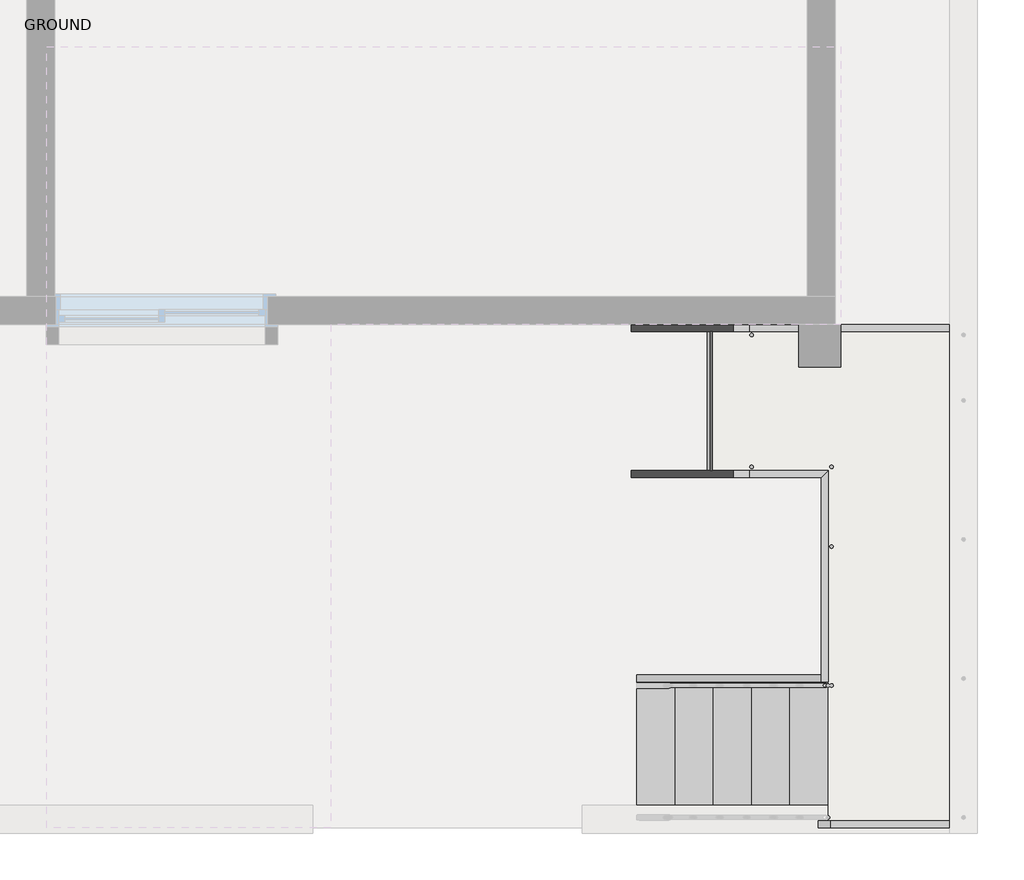
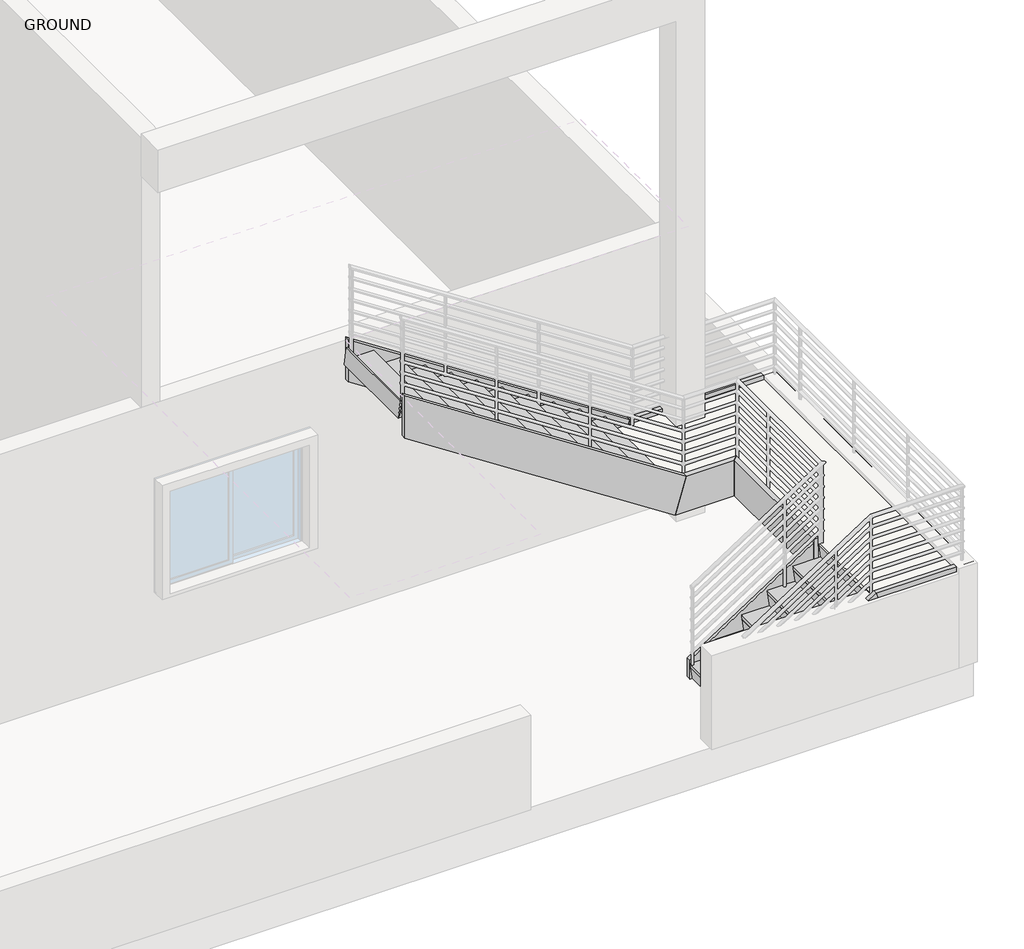
# One storey, part 4 of 4: 9 members, 2 stair flights, 1 slab.
"""IFC4 building model written with IfcOpenShell, lengths in millimetres."""

from ifc_helpers import new_model, si_unit, frame, origin, place, context, project, spatial, polyline, outline, extrude, faceted_brep, transform, mapped, element, save
from components import non_monolithic_landing_a96adf93, stair_flight_50mm_tread_25mm_nosing_13mm_riser_d89b79ae, stair_flight_50mm_tread_25mm_nosing_13mm_riser_9fd7d1ab

model = new_model("IFC4")

# Units and contexts
model_context = context("Model", 3, world=origin())
ifc_project = project(units=[si_unit("LENGTHUNIT", "METRE", prefix="MILLI")], contexts=[model_context])

# Site, building, storey
site = spatial("IfcSite", under=ifc_project)
building = spatial("IfcBuilding", under=site)
storey = spatial("IfcBuildingStorey", under=building, Name="GROUND", Elevation=0.0)

# Members
placement = place(None, origin())
element("IfcMember", 1, ObjectType="Stringer - 50mm Width", at=placement, inside=storey, context=model_context, shape_type="SweptSolid", body=[
    extrude(outline(polyline([(216.9803521, 11825.7864069), (0.0, 11825.7864069), (0.0, 12225.3790476), (603.3458035, 13150.7864069), (1080.8520099, 13150.7864069), (216.9803521, 11825.7864069)])), frame((0.0, -2533.727917, 0.0), z_axis=(0.0, 1.0, 0.0), x_axis=(0.0, 0.0, 1.0)), (0.0, 0.0, 1.0), 50.0),
])
element("IfcMember", 2, ObjectType="Stringer - 50mm Width", at=placement, inside=storey, context=model_context, shape_type="SweptSolid", body=[
    extrude(outline(polyline([(216.9803521, 11825.7864069), (0.0, 11825.7864069), (0.0, 12225.3790476), (723.1584328, 13334.5541373), (1123.1584328, 13215.6756875), (216.9803521, 11825.7864069)])), frame((0.0, -3583.7536983, 0.0), z_axis=(0.0, 1.0, 0.0), x_axis=(0.0, 0.0, 1.0)), (0.0, 0.0, 1.0), 50.0),
])
element("IfcMember", 3, ObjectType="Stringer - 50mm Width", at=placement, inside=storey, context=model_context, shape_type="SweptSolid", body=[
    extrude(outline(polyline([(723.1584328, 12517.0186765), (1123.1584328, 12635.8971263), (3085.6862345, 9625.7864069), (2608.1800281, 9625.7864069), (723.1584328, 12517.0186765)])), frame((0.0, -1061.9101069, 0.0), z_axis=(0.0, 1.0, 0.0), x_axis=(0.0, 0.0, 1.0)), (0.0, 0.0, 1.0), 50.0),
])
element("IfcMember", 4, ObjectType="Stringer - 50mm Width", at=placement, inside=storey, context=model_context, shape_type="SweptSolid", body=[
    extrude(outline(polyline([(723.1584328, 12517.0186765), (1123.1584328, 12635.8971263), (3085.6862345, 9625.7864069), (2608.1800281, 9625.7864069), (723.1584328, 12517.0186765)])), frame((0.0, -11.8843256, 0.0), z_axis=(0.0, 1.0, 0.0), x_axis=(0.0, 0.0, 1.0)), (0.0, 0.0, 1.0), 50.0),
])
element("IfcMember", 5, ObjectType="Stringer - 50mm Width", at=placement, inside=storey, context=model_context, shape_type="Brep", body=[
    faceted_brep([(12635.8971263, -1011.9101069, 1123.1584328), (12635.8971263, -1061.9101069, 1123.1584328), (13150.7864069, -1061.9101069, 1123.1584328), (13200.7864069, -1011.9101069, 1123.1584328), (12517.0186765, -1011.9101069, 723.1584328), (13200.7864069, -1011.9101069, 723.1584328), (12517.0186765, -1061.9101069, 723.1584328), (13150.7864069, -1061.9101069, 723.1584328)], [[[0, 1, 2, 3]], [[4, 0, 3, 5]], [[6, 4, 5, 7]], [[1, 6, 7, 2]], [[1, 0, 4, 6]], [[2, 7, 5, 3]]]),
])
element("IfcMember", 6, ObjectType="Stringer - 50mm Width", at=placement, inside=storey, context=model_context, shape_type="SweptSolid", body=[
    extrude(outline(polyline([(13150.7864069, -1061.9101069), (13200.7864069, -1011.9101069), (13200.7864069, -2533.727917), (13150.7864069, -2533.727917), (13150.7864069, -1061.9101069)])), frame((0.0, 0.0, 723.1584328), z_axis=(0.0, 0.0, 1.0), x_axis=(1.0, 0.0, 0.0)), (0.0, 0.0, 1.0), 400.0),
])
element("IfcMember", 7, ObjectType="Stringer - 50mm Width", at=placement, inside=storey, context=model_context, shape_type="Brep", body=[
    faceted_brep([(13215.6756875, -3533.7536983, 1123.1584328), (13215.6756875, -3583.7536983, 1123.1584328), (14250.8121881, -3583.7536983, 1123.1584328), (14200.8121881, -3533.7536983, 1123.1584328), (13334.5541373, -3533.7536983, 723.1584328), (14200.8121881, -3533.7536983, 723.1584328), (13334.5541373, -3583.7536983, 723.1584328), (14250.8121881, -3583.7536983, 723.1584328)], [[[0, 1, 2, 3]], [[4, 0, 3, 5]], [[6, 4, 5, 7]], [[1, 6, 7, 2]], [[1, 0, 4, 6]], [[2, 7, 5, 3]]]),
])
element("IfcMember", 8, ObjectType="Stringer - 50mm Width", at=placement, inside=storey, context=model_context, shape_type="SweptSolid", body=[
    extrude(outline(polyline([(14250.8121881, -3583.7536983), (14200.8121881, -3533.7536983), (14200.8121881, -11.8843256), (14250.8121881, 38.1156744), (14250.8121881, -3583.7536983)])), frame((0.0, 0.0, 723.1584328), z_axis=(0.0, 0.0, 1.0), x_axis=(1.0, 0.0, 0.0)), (0.0, 0.0, 1.0), 400.0),
])
element("IfcMember", 9, ObjectType="Stringer - 50mm Width", at=placement, inside=storey, context=model_context, shape_type="Brep", body=[
    faceted_brep([(14200.8121881, -11.8843256, 1123.1584328), (14250.8121881, 38.1156744, 1123.1584328), (12635.8971263, 38.1156744, 1123.1584328), (12635.8971263, -11.8843256, 1123.1584328), (14200.8121881, -11.8843256, 723.1584328), (12517.0186765, -11.8843256, 723.1584328), (14250.8121881, 38.1156744, 723.1584328), (12517.0186765, 38.1156744, 723.1584328)], [[[0, 1, 2, 3]], [[4, 0, 3, 5]], [[6, 4, 5, 7]], [[1, 6, 7, 2]], [[1, 0, 4, 6]], [[2, 7, 5, 3]]]),
])

# Slab
non_monolithic_landing_shape = non_monolithic_landing_a96adf93(model_context)
element("IfcSlab", 10, ObjectType="Non-Monolithic Landing", at=placement, inside=storey, context=model_context, shape_type="MappedRepresentation", body=[
    mapped(non_monolithic_landing_shape, transform((0.0, 0.0, 0.0), x_axis=(1.0, 0.0, 0.0), y_axis=(0.0, 1.0, 0.0), z_axis=(0.0, 0.0, 1.0))),
])

# Stair flights
stair_flight_50mm_tread_25mm_nosing_13mm_riser_shape = stair_flight_50mm_tread_25mm_nosing_13mm_riser_d89b79ae(model_context)
element("IfcStairFlight", 11, ObjectType="50mm Tread 25mm Nosing 13mm Riser", at=placement, inside=storey, context=model_context, shape_type="MappedRepresentation", body=[
    mapped(stair_flight_50mm_tread_25mm_nosing_13mm_riser_shape, transform((0.0, 0.0, 0.0), x_axis=(1.0, 0.0, 0.0), y_axis=(0.0, 1.0, 0.0), z_axis=(0.0, 0.0, 1.0))),
])
stair_flight_50mm_tread_25mm_nosing_13mm_riser_2_shape = stair_flight_50mm_tread_25mm_nosing_13mm_riser_9fd7d1ab(model_context)
element("IfcStairFlight", 12, ObjectType="50mm Tread 25mm Nosing 13mm Riser", at=placement, inside=storey, context=model_context, shape_type="MappedRepresentation", body=[
    mapped(stair_flight_50mm_tread_25mm_nosing_13mm_riser_2_shape, transform((0.0, 0.0, 0.0), x_axis=(1.0, 0.0, 0.0), y_axis=(0.0, 1.0, 0.0), z_axis=(0.0, 0.0, 1.0))),
])

save(model, "model.ifc")

# Revit data of these elements
# Elements 1, 2, 3, 4, 5, 6, 7, 8, 9 (IfcMember, "Stringer - 50mm Width")
#   Phase Created = New Construction
# Element 10 (IfcSlab, "Non-Monolithic Landing")
#   Phase Created = New Construction
# Elements 11, 12 (IfcStairFlight, "50mm Tread 25mm Nosing 13mm Riser")
#   Phase Created = New Construction
